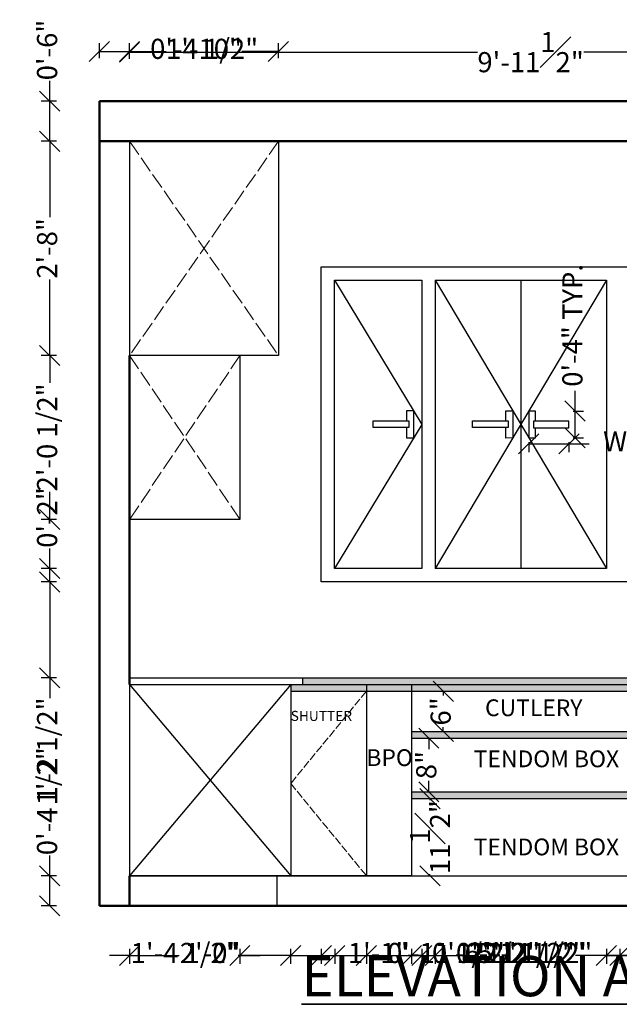
# Model space of a CAD drawing. Units: inches. Extents: x 2164 to 2316, y 625 to 771.
# Tile 1 of 2: x 2164 to 2253, y 625 to 771. Entities that reach past the tile are written whole.
import ezdxf

# ---------------------------------------------------------------- set-up
doc = ezdxf.new("R2010")
doc.units = ezdxf.units.IN
doc.linetypes.add('ACAD_ISO02W100', pattern=[15, 12, -3])
for name, color, linetype, lineweight in [('A-ANNO-DIMS', 2, 'Continuous', 18), ('A-ANNO-TEXT', 7, 'Continuous', 18), ('A-ANNO-TTLB', 7, 'Continuous', 35), ('A-FURN', 30, 'Continuous', 25), ('A-FURN-OPEN', 8, 'ACAD_ISO02W100', 13), ('A-FURN-PATT', 8, 'Continuous', 13), ('A-GLAZ', 4, 'Continuous', 25), ('A-WALL', 7, 'Continuous', 50)]:
    doc.layers.add(name, color=color, linetype=linetype, lineweight=lineweight)
doc.styles.get("Standard").update_dxf_attribs({"font": 'arial.ttf'})
doc.dimstyles.new('ISO-25', dxfattribs={"dimtxt": 3, "dimasz": 3, "dimexe": 1.25, "dimexo": 0.625, "dimtad": 0, "dimdec": 5, "dimlunit": 4, "dimtxsty": 'Standard', "dimblk": 'OBLIQUE', "dimcen": 2.5, "dimclrt": 1, "dimadec": 0, "dimazin": 0, "dimtfac": 1, "dimtdec": 5, "dimtmove": 0, "dimatfit": 3, "dimldrblk": 'OBLIQUE', "dimfxl": 1, "dimfxlon": 1, "dimfrac": 1, "dimarcsym": 0})

# ---------------------------------------------------------------- blocks, each defined once
blk = doc.blocks.new('_Oblique')
at = {"color": 0, "linetype": 'ByBlock', "lineweight": -2}
blk.add_line((-0.5, -0.5), (0.5, 0.5), dxfattribs=at)
blk = doc.blocks.new('*D1')
at = {"layer": 'A-ANNO-DIMS', "color": 0, "lineweight": -2, "transparency": 16777216}
for p, q in [((2226.19, 671.25), (2228.44, 671.25)), ((2227.19, 671.25), (2227.19, 670.61)), ((2226.19, 665.25), (2228.44, 665.25)), ((2227.19, 665.25), (2227.19, 665.9))]:
    blk.add_line(p, q, dxfattribs=at)
at = {"layer": 'Defpoints', "color": 0, "transparency": 16777216}
for p in [(2222.45, 671.25), (2222.45, 665.25), (2227.19, 665.25)]:
    blk.add_point(p, dxfattribs=at)
at = {"layer": 'A-ANNO-DIMS', "color": 0, "lineweight": -2, "transparency": 16777216, "xscale": 3, "yscale": 3, "zscale": 3}
for p, rotation in [((2227.19, 671.25), 90), ((2227.19, 665.25), 270)]:
    blk.add_blockref('_Oblique', p, dxfattribs=dict(at, rotation=rotation))
at = {"layer": 'A-ANNO-DIMS', "color": 0, "transparency": 16777216, "insert": (2227.19, 668.25), "char_height": 3, "attachment_point": 5, "rotation": 90}
blk.add_mtext('6"', dxfattribs=at)
blk = doc.blocks.new('*D2')
at = {"layer": 'A-ANNO-DIMS', "color": 0, "lineweight": -2, "transparency": 16777216}
for p, q in [((2224.04, 664.25), (2226.29, 664.25)), ((2225.04, 664.25), (2225.04, 662.6)), ((2225.04, 656.25), (2225.04, 657.9)), ((2224.04, 656.25), (2226.29, 656.25))]:
    blk.add_line(p, q, dxfattribs=at)
at = {"layer": 'Defpoints', "color": 0, "transparency": 16777216}
for p in [(2222.45, 664.25), (2222.45, 656.25), (2225.04, 656.25)]:
    blk.add_point(p, dxfattribs=at)
at = {"layer": 'A-ANNO-DIMS', "color": 0, "lineweight": -2, "transparency": 16777216, "xscale": 3, "yscale": 3, "zscale": 3}
for p, rotation in [((2225.04, 664.25), 90), ((2225.04, 656.25), 270)]:
    blk.add_blockref('_Oblique', p, dxfattribs=dict(at, rotation=rotation))
at = {"layer": 'A-ANNO-DIMS', "color": 0, "transparency": 16777216, "insert": (2225.04, 660.25), "char_height": 3, "attachment_point": 5, "rotation": 90}
blk.add_mtext('8"', dxfattribs=at)
blk = doc.blocks.new('*D3')
at = {"layer": 'A-ANNO-DIMS', "color": 0, "lineweight": -2, "transparency": 16777216}
for p, q in [((2224.21, 655.25), (2226.46, 655.25)), ((2225.21, 655.25), (2225.21, 655.02)), ((2224.21, 643.75), (2226.46, 643.75)), ((2225.21, 643.75), (2225.21, 643.98))]:
    blk.add_line(p, q, dxfattribs=at)
at = {"layer": 'Defpoints', "color": 0, "transparency": 16777216}
for p in [(2222.45, 655.25), (2222.45, 643.75), (2225.21, 643.75)]:
    blk.add_point(p, dxfattribs=at)
at = {"layer": 'A-ANNO-DIMS', "color": 0, "lineweight": -2, "transparency": 16777216, "xscale": 3, "yscale": 3, "zscale": 3}
for p, rotation in [((2225.21, 655.25), 90), ((2225.21, 643.75), 270)]:
    blk.add_blockref('_Oblique', p, dxfattribs=dict(at, rotation=rotation))
at = {"layer": 'A-ANNO-DIMS', "color": 0, "transparency": 16777216, "insert": (2225.21, 649.5), "char_height": 3, "attachment_point": 5, "rotation": 90}
blk.add_mtext('11{\\H1x;\\S1#2;}"', dxfattribs=at)
blk = doc.blocks.new('*D4')
at = {"layer": 'A-ANNO-DIMS', "color": 0, "lineweight": -2, "transparency": 16777216}
for p, q in [((2180.45, 765.55), (2180.45, 767.8)), ((2299.95, 765.55), (2299.95, 767.8)), ((2180.45, 766.55), (2232.28, 766.55)), ((2299.95, 766.55), (2248.13, 766.55))]:
    blk.add_line(p, q, dxfattribs=at)
at = {"layer": 'Defpoints', "color": 0, "transparency": 16777216}
for p in [(2299.95, 766.55), (2180.45, 759.25), (2299.95, 759.25)]:
    blk.add_point(p, dxfattribs=at)
at = {"layer": 'A-ANNO-DIMS', "color": 0, "lineweight": -2, "transparency": 16777216, "xscale": 3, "yscale": 3, "zscale": 3, "rotation": 180}
blk.add_blockref('_Oblique', (2180.45, 766.55), dxfattribs=at)
at = {"layer": 'A-ANNO-DIMS', "color": 0, "lineweight": -2, "transparency": 16777216, "xscale": 3, "yscale": 3, "zscale": 3}
blk.add_blockref('_Oblique', (2299.95, 766.55), dxfattribs=at)
at = {"layer": 'A-ANNO-DIMS', "color": 0, "transparency": 16777216, "insert": (2240.2, 766.55), "char_height": 3, "attachment_point": 5}
blk.add_mtext('9\'-11{\\H1x;\\S1#2;}"', dxfattribs=at)
blk = doc.blocks.new('WIN-HANDLE')
blk.add_lwpolyline([(2239.92, 710.04), (2239.92, 709.04), (2240.92, 709.04), (2240.92, 710.54), (2245.92, 710.54), (2245.92, 711.54), (2240.92, 711.54), (2240.92, 713.04), (2239.92, 713.04), (2239.92, 711.04)], close=True)
blk.add_lwpolyline([(2240.92, 711.54), (2240.62, 711.54), (2240.62, 710.54), (2240.92, 710.54)])
blk = doc.blocks.new('*D8')
at = {"layer": 'A-ANNO-DIMS', "color": 0, "lineweight": -2, "transparency": 16777216}
for p, q in [((2239.92, 708.42), (2239.92, 706.89)), ((2239.92, 708.14), (2245.92, 708.14)), ((2245.92, 708.42), (2245.92, 706.89)), ((2245.92, 708.14), (2248.92, 708.14))]:
    blk.add_line(p, q, dxfattribs=at)
at = {"layer": 'Defpoints', "color": 0, "transparency": 16777216}
for p in [(2239.92, 709.04), (2245.92, 709.04), (2245.92, 708.14)]:
    blk.add_point(p, dxfattribs=at)
at = {"layer": 'A-ANNO-DIMS', "color": 0, "lineweight": -2, "transparency": 16777216, "xscale": 3, "yscale": 3, "zscale": 3, "rotation": 180}
blk.add_blockref('_Oblique', (2239.92, 708.14), dxfattribs=at)
at = {"layer": 'A-ANNO-DIMS', "color": 0, "lineweight": -2, "transparency": 16777216, "xscale": 3, "yscale": 3, "zscale": 3}
blk.add_blockref('_Oblique', (2245.92, 708.14), dxfattribs=at)
at = {"layer": 'A-ANNO-DIMS', "color": 1, "transparency": 16777216, "insert": (2277.61, 708.14), "char_height": 3, "attachment_point": 5}
blk.add_mtext('WINDOW HANDLE 0\'-6" TYP.', dxfattribs=at)
blk = doc.blocks.new('*D9')
at = {"layer": 'A-ANNO-DIMS', "color": 0, "lineweight": -2, "transparency": 16777216}
for p, q in [((2246.82, 713.04), (2246.82, 716.04)), ((2246.55, 713.04), (2248.07, 713.04)), ((2246.82, 709.04), (2246.82, 713.04)), ((2246.55, 709.04), (2248.07, 709.04))]:
    blk.add_line(p, q, dxfattribs=at)
at = {"layer": 'Defpoints', "color": 0, "transparency": 16777216}
for p in [(2245.92, 713.04), (2246.82, 713.04), (2245.92, 709.04)]:
    blk.add_point(p, dxfattribs=at)
at = {"layer": 'A-ANNO-DIMS', "color": 0, "lineweight": -2, "transparency": 16777216, "xscale": 3, "yscale": 3, "zscale": 3}
for p, rotation in [((2246.82, 713.04), 90), ((2246.82, 709.04), 270)]:
    blk.add_blockref('_Oblique', p, dxfattribs=dict(at, rotation=rotation))
at = {"layer": 'A-ANNO-DIMS', "color": 1, "transparency": 16777216, "insert": (2246.82, 725.81), "char_height": 3, "attachment_point": 5, "rotation": 90}
blk.add_mtext('0\'-4" TYP.', dxfattribs=at)
blk = doc.blocks.new('*D10')
at = {"layer": 'A-ANNO-DIMS', "color": 0, "lineweight": -2, "transparency": 16777216}
for p, q in [((2180.45, 765.65), (2180.45, 767.9)), ((2202.62, 765.65), (2202.62, 767.9)), ((2180.45, 766.65), (2185.9, 766.65)), ((2202.62, 766.65), (2197.17, 766.65))]:
    blk.add_line(p, q, dxfattribs=at)
at = {"layer": 'Defpoints', "color": 0, "transparency": 16777216}
for p in [(2202.62, 766.65), (2180.45, 753.25), (2202.62, 753.25)]:
    blk.add_point(p, dxfattribs=at)
at = {"layer": 'A-ANNO-DIMS', "color": 0, "lineweight": -2, "transparency": 16777216, "xscale": 3, "yscale": 3, "zscale": 3, "rotation": 180}
blk.add_blockref('_Oblique', (2180.45, 766.65), dxfattribs=at)
at = {"layer": 'A-ANNO-DIMS', "color": 0, "lineweight": -2, "transparency": 16777216, "xscale": 3, "yscale": 3, "zscale": 3}
blk.add_blockref('_Oblique', (2202.62, 766.65), dxfattribs=at)
at = {"layer": 'A-ANNO-DIMS', "color": 1, "transparency": 16777216, "insert": (2191.54, 766.65), "char_height": 3, "attachment_point": 5}
blk.add_mtext('1\'-10"', dxfattribs=at)
blk = doc.blocks.new('*D12')
at = {"layer": 'A-ANNO-DIMS', "color": 0, "lineweight": -2, "transparency": 16777216}
for p, q in [((2169.55, 753.25), (2167.3, 753.25)), ((2168.55, 753.25), (2168.55, 741.93)), ((2168.55, 721.33), (2168.55, 732.65)), ((2169.55, 721.33), (2167.3, 721.33))]:
    blk.add_line(p, q, dxfattribs=at)
at = {"layer": 'Defpoints', "color": 0, "transparency": 16777216}
for p in [(2180.45, 753.25), (2168.55, 721.33), (2180.45, 721.33)]:
    blk.add_point(p, dxfattribs=at)
at = {"layer": 'A-ANNO-DIMS', "color": 0, "lineweight": -2, "transparency": 16777216, "xscale": 3, "yscale": 3, "zscale": 3}
for p, rotation in [((2168.55, 753.25), 90), ((2168.55, 721.33), 270)]:
    blk.add_blockref('_Oblique', p, dxfattribs=dict(at, rotation=rotation))
at = {"layer": 'A-ANNO-DIMS', "color": 1, "transparency": 16777216, "insert": (2168.55, 737.29), "char_height": 3, "attachment_point": 5, "rotation": 90}
blk.add_mtext('2\'-8"', dxfattribs=at)
blk = doc.blocks.new('*D13')
at = {"layer": 'A-ANNO-DIMS', "color": 0, "lineweight": -2, "transparency": 16777216}
for p, q in [((2169.55, 721.33), (2167.3, 721.33)), ((2168.55, 721.33), (2168.55, 717.24)), ((2168.55, 696.88), (2168.55, 700.97)), ((2169.55, 696.88), (2167.3, 696.88))]:
    blk.add_line(p, q, dxfattribs=at)
at = {"layer": 'Defpoints', "color": 0, "transparency": 16777216}
for p in [(2180.45, 721.33), (2168.55, 696.88), (2180.45, 696.88)]:
    blk.add_point(p, dxfattribs=at)
at = {"layer": 'A-ANNO-DIMS', "color": 0, "lineweight": -2, "transparency": 16777216, "xscale": 3, "yscale": 3, "zscale": 3}
for p, rotation in [((2168.55, 721.33), 90), ((2168.55, 696.88), 270)]:
    blk.add_blockref('_Oblique', p, dxfattribs=dict(at, rotation=rotation))
at = {"layer": 'A-ANNO-DIMS', "color": 1, "transparency": 16777216, "insert": (2168.55, 709.11), "char_height": 3, "attachment_point": 5, "rotation": 90}
blk.add_mtext('2\'-0 1/2"', dxfattribs=at)
blk = doc.blocks.new('*D14')
at = {"layer": 'A-ANNO-DIMS', "color": 0, "lineweight": -2, "transparency": 16777216}
for p, q in [((2180.45, 632.85), (2180.45, 630.6)), ((2196.89, 632.85), (2196.89, 630.6)), ((2180.45, 631.85), (2177.45, 631.85)), ((2180.45, 631.85), (2180.71, 631.85)), ((2196.89, 631.85), (2196.64, 631.85)), ((2196.89, 631.85), (2199.89, 631.85))]:
    blk.add_line(p, q, dxfattribs=at)
at = {"layer": 'Defpoints', "color": 0, "transparency": 16777216}
for p in [(2180.45, 696.88), (2196.89, 696.88), (2196.89, 631.85)]:
    blk.add_point(p, dxfattribs=at)
at = {"layer": 'A-ANNO-DIMS', "color": 0, "lineweight": -2, "transparency": 16777216, "xscale": 3, "yscale": 3, "zscale": 3}
blk.add_blockref('_Oblique', (2180.45, 631.85), dxfattribs=at)
at = {"layer": 'A-ANNO-DIMS', "color": 0, "lineweight": -2, "transparency": 16777216, "xscale": 3, "yscale": 3, "zscale": 3, "rotation": 180}
blk.add_blockref('_Oblique', (2196.89, 631.85), dxfattribs=at)
at = {"layer": 'A-ANNO-DIMS', "color": 1, "transparency": 16777216, "insert": (2188.67, 631.85), "char_height": 3, "attachment_point": 5}
blk.add_mtext('1\'-4 1/2"', dxfattribs=at)
blk = doc.blocks.new('*D17')
at = {"layer": 'A-ANNO-DIMS', "color": 0, "lineweight": -2, "transparency": 16777216}
for p, q in [((2211.01, 632.85), (2211.01, 630.6)), ((2223.98, 632.85), (2223.98, 630.6)), ((2211.01, 631.85), (2213.02, 631.85)), ((2223.98, 631.85), (2221.96, 631.85))]:
    blk.add_line(p, q, dxfattribs=at)
at = {"layer": 'Defpoints', "color": 0, "transparency": 16777216}
for p in [(2211.01, 689.55), (2223.98, 689.55), (2223.98, 631.85)]:
    blk.add_point(p, dxfattribs=at)
at = {"layer": 'A-ANNO-DIMS', "color": 0, "lineweight": -2, "transparency": 16777216, "xscale": 3, "yscale": 3, "zscale": 3, "rotation": 180}
blk.add_blockref('_Oblique', (2211.01, 631.85), dxfattribs=at)
at = {"layer": 'A-ANNO-DIMS', "color": 0, "lineweight": -2, "transparency": 16777216, "xscale": 3, "yscale": 3, "zscale": 3}
blk.add_blockref('_Oblique', (2223.98, 631.85), dxfattribs=at)
at = {"layer": 'A-ANNO-DIMS', "color": 1, "transparency": 16777216, "insert": (2217.49, 631.85), "char_height": 3, "attachment_point": 5}
blk.add_mtext('1\'-1"', dxfattribs=at)
blk = doc.blocks.new('*D18')
at = {"layer": 'A-ANNO-DIMS', "color": 0, "lineweight": -2, "transparency": 16777216}
for p, q in [((2223.98, 632.85), (2223.98, 630.6)), ((2225.98, 632.85), (2225.98, 630.6)), ((2223.98, 631.85), (2225.98, 631.85)), ((2225.98, 631.85), (2228.98, 631.85))]:
    blk.add_line(p, q, dxfattribs=at)
at = {"layer": 'Defpoints', "color": 0, "transparency": 16777216}
for p in [(2223.98, 689.55), (2225.98, 689.55), (2225.98, 631.85)]:
    blk.add_point(p, dxfattribs=at)
at = {"layer": 'A-ANNO-DIMS', "color": 0, "lineweight": -2, "transparency": 16777216, "xscale": 3, "yscale": 3, "zscale": 3, "rotation": 180}
blk.add_blockref('_Oblique', (2223.98, 631.85), dxfattribs=at)
at = {"layer": 'A-ANNO-DIMS', "color": 0, "lineweight": -2, "transparency": 16777216, "xscale": 3, "yscale": 3, "zscale": 3}
blk.add_blockref('_Oblique', (2225.98, 631.85), dxfattribs=at)
at = {"layer": 'A-ANNO-DIMS', "color": 1, "transparency": 16777216, "insert": (2233.59, 631.85), "char_height": 3, "attachment_point": 5}
blk.add_mtext('0\'-2"', dxfattribs=at)
blk = doc.blocks.new('*D19')
at = {"layer": 'A-ANNO-DIMS', "color": 0, "lineweight": -2, "transparency": 16777216}
for p, q in [((2225.98, 632.85), (2225.98, 630.6)), ((2251.49, 632.85), (2251.49, 630.6)), ((2225.98, 631.85), (2230.6, 631.85)), ((2251.49, 631.85), (2246.87, 631.85))]:
    blk.add_line(p, q, dxfattribs=at)
at = {"layer": 'Defpoints', "color": 0, "transparency": 16777216}
for p in [(2225.98, 689.55), (2251.49, 689.55), (2251.49, 631.85)]:
    blk.add_point(p, dxfattribs=at)
at = {"layer": 'A-ANNO-DIMS', "color": 0, "lineweight": -2, "transparency": 16777216, "xscale": 3, "yscale": 3, "zscale": 3, "rotation": 180}
blk.add_blockref('_Oblique', (2225.98, 631.85), dxfattribs=at)
at = {"layer": 'A-ANNO-DIMS', "color": 0, "lineweight": -2, "transparency": 16777216, "xscale": 3, "yscale": 3, "zscale": 3}
blk.add_blockref('_Oblique', (2251.49, 631.85), dxfattribs=at)
at = {"layer": 'A-ANNO-DIMS', "color": 1, "transparency": 16777216, "insert": (2238.74, 631.85), "char_height": 3, "attachment_point": 5}
blk.add_mtext('2\'-1 1/2"', dxfattribs=at)
blk = doc.blocks.new('*D20')
at = {"layer": 'A-ANNO-DIMS', "color": 0, "lineweight": -2, "transparency": 16777216}
for p, q in [((2251.49, 632.85), (2251.49, 630.6)), ((2253.49, 632.85), (2253.49, 630.6)), ((2251.49, 631.85), (2253.49, 631.85)), ((2253.49, 631.85), (2256.49, 631.85))]:
    blk.add_line(p, q, dxfattribs=at)
at = {"layer": 'Defpoints', "color": 0, "transparency": 16777216}
for p in [(2251.49, 689.55), (2253.49, 689.55), (2253.49, 631.85)]:
    blk.add_point(p, dxfattribs=at)
at = {"layer": 'A-ANNO-DIMS', "color": 0, "lineweight": -2, "transparency": 16777216, "xscale": 3, "yscale": 3, "zscale": 3, "rotation": 180}
blk.add_blockref('_Oblique', (2251.49, 631.85), dxfattribs=at)
at = {"layer": 'A-ANNO-DIMS', "color": 0, "lineweight": -2, "transparency": 16777216, "xscale": 3, "yscale": 3, "zscale": 3}
blk.add_blockref('_Oblique', (2253.49, 631.85), dxfattribs=at)
at = {"layer": 'A-ANNO-DIMS', "color": 1, "transparency": 16777216, "insert": (2261.11, 631.85), "char_height": 3, "attachment_point": 5}
blk.add_mtext('0\'-2"', dxfattribs=at)
blk = doc.blocks.new('*D21')
at = {"layer": 'A-ANNO-DIMS', "color": 0, "lineweight": -2, "transparency": 16777216}
for p, q in [((2253.49, 632.85), (2253.49, 630.6)), ((2269.66, 632.85), (2269.66, 630.6)), ((2253.49, 631.85), (2257.11, 631.85)), ((2269.66, 631.85), (2266.05, 631.85))]:
    blk.add_line(p, q, dxfattribs=at)
at = {"layer": 'Defpoints', "color": 0, "transparency": 16777216}
for p in [(2253.49, 689.55), (2269.66, 689.55), (2269.66, 631.85)]:
    blk.add_point(p, dxfattribs=at)
at = {"layer": 'A-ANNO-DIMS', "color": 0, "lineweight": -2, "transparency": 16777216, "xscale": 3, "yscale": 3, "zscale": 3, "rotation": 180}
blk.add_blockref('_Oblique', (2253.49, 631.85), dxfattribs=at)
at = {"layer": 'A-ANNO-DIMS', "color": 0, "lineweight": -2, "transparency": 16777216, "xscale": 3, "yscale": 3, "zscale": 3}
blk.add_blockref('_Oblique', (2269.66, 631.85), dxfattribs=at)
at = {"layer": 'A-ANNO-DIMS', "color": 1, "transparency": 16777216, "insert": (2261.58, 631.85), "char_height": 3, "attachment_point": 5}
blk.add_mtext('1\'-4"', dxfattribs=at)
blk = doc.blocks.new('*D23')
at = {"layer": 'A-ANNO-DIMS', "color": 0, "lineweight": -2, "transparency": 16777216}
for p, q in [((2209.01, 632.85), (2209.01, 630.6)), ((2271.66, 632.85), (2271.66, 630.6)), ((2209.01, 631.85), (2232.23, 631.85)), ((2271.66, 631.85), (2248.44, 631.85))]:
    blk.add_line(p, q, dxfattribs=at)
at = {"layer": 'Defpoints', "color": 0, "transparency": 16777216}
for p in [(2209.01, 687.55), (2271.66, 687.55), (2271.66, 631.85)]:
    blk.add_point(p, dxfattribs=at)
at = {"layer": 'A-ANNO-DIMS', "color": 0, "lineweight": -2, "transparency": 16777216, "xscale": 3, "yscale": 3, "zscale": 3, "rotation": 180}
blk.add_blockref('_Oblique', (2209.01, 631.85), dxfattribs=at)
at = {"layer": 'A-ANNO-DIMS', "color": 0, "lineweight": -2, "transparency": 16777216, "xscale": 3, "yscale": 3, "zscale": 3}
blk.add_blockref('_Oblique', (2271.66, 631.85), dxfattribs=at)
at = {"layer": 'A-ANNO-DIMS', "color": 1, "transparency": 16777216, "insert": (2240.33, 631.85), "char_height": 3, "attachment_point": 5}
blk.add_mtext('5\'-2 1/2"', dxfattribs=at)
blk = doc.blocks.new('*D25')
at = {"layer": 'A-ANNO-DIMS', "color": 0, "lineweight": -2, "transparency": 16777216}
for p, q in [((2168.55, 689.55), (2168.55, 692.55)), ((2169.55, 689.55), (2167.3, 689.55)), ((2168.55, 687.55), (2168.55, 689.55)), ((2169.55, 687.55), (2167.3, 687.55))]:
    blk.add_line(p, q, dxfattribs=at)
at = {"layer": 'Defpoints', "color": 0, "transparency": 16777216}
for p in [(2168.55, 689.55), (2211.01, 689.55), (2209.01, 687.55)]:
    blk.add_point(p, dxfattribs=at)
at = {"layer": 'A-ANNO-DIMS', "color": 0, "lineweight": -2, "transparency": 16777216, "xscale": 3, "yscale": 3, "zscale": 3}
for p, rotation in [((2168.55, 689.55), 90), ((2168.55, 687.55), 270)]:
    blk.add_blockref('_Oblique', p, dxfattribs=dict(at, rotation=rotation))
at = {"layer": 'A-ANNO-DIMS', "color": 1, "transparency": 16777216, "insert": (2168.55, 697.16), "char_height": 3, "attachment_point": 5, "rotation": 90}
blk.add_mtext('0\'-2"', dxfattribs=at)
blk = doc.blocks.new('*D29')
at = {"layer": 'A-ANNO-DIMS', "color": 0, "lineweight": -2, "transparency": 16777216}
for p, q in [((2169.55, 687.55), (2167.3, 687.55)), ((2168.55, 687.55), (2168.55, 673.25)), ((2169.55, 673.25), (2167.3, 673.25)), ((2168.55, 673.25), (2168.55, 670.25))]:
    blk.add_line(p, q, dxfattribs=at)
at = {"layer": 'Defpoints', "color": 0, "transparency": 16777216}
for p in [(2209.01, 687.55), (2168.55, 673.25), (2180.45, 673.25)]:
    blk.add_point(p, dxfattribs=at)
at = {"layer": 'A-ANNO-DIMS', "color": 0, "lineweight": -2, "transparency": 16777216, "xscale": 3, "yscale": 3, "zscale": 3}
for p, rotation in [((2168.55, 687.55), 90), ((2168.55, 673.25), 270)]:
    blk.add_blockref('_Oblique', p, dxfattribs=dict(at, rotation=rotation))
at = {"layer": 'A-ANNO-DIMS', "color": 1, "transparency": 16777216, "insert": (2168.55, 662.29), "char_height": 3, "attachment_point": 5, "rotation": 90}
blk.add_mtext('1\'-2 1/2"', dxfattribs=at)
blk = doc.blocks.new('*D34')
at = {"layer": 'A-ANNO-DIMS', "color": 0, "lineweight": -2, "transparency": 16777216}
for p, q in [((2168.55, 643.75), (2168.55, 646.75)), ((2169.55, 643.75), (2167.3, 643.75)), ((2168.55, 639.25), (2168.55, 643.75)), ((2169.55, 639.25), (2167.3, 639.25))]:
    blk.add_line(p, q, dxfattribs=at)
at = {"layer": 'Defpoints', "color": 0, "transparency": 16777216}
for p in [(2168.55, 643.75), (2180.45, 643.75), (2180.45, 639.25)]:
    blk.add_point(p, dxfattribs=at)
at = {"layer": 'A-ANNO-DIMS', "color": 0, "lineweight": -2, "transparency": 16777216, "xscale": 3, "yscale": 3, "zscale": 3}
for p, rotation in [((2168.55, 643.75), 90), ((2168.55, 639.25), 270)]:
    blk.add_blockref('_Oblique', p, dxfattribs=dict(at, rotation=rotation))
at = {"layer": 'A-ANNO-DIMS', "color": 1, "transparency": 16777216, "insert": (2168.55, 654.86), "char_height": 3, "attachment_point": 5, "rotation": 90}
blk.add_mtext('0\'-4 1/2"', dxfattribs=at)
blk = doc.blocks.new('*D35')
at = {"layer": 'A-ANNO-DIMS', "color": 0, "lineweight": -2, "transparency": 16777216}
for p, q in [((2180.45, 632.85), (2180.45, 630.6)), ((2204.45, 632.85), (2204.45, 630.6)), ((2180.45, 631.85), (2187.82, 631.85)), ((2204.45, 631.85), (2197.09, 631.85))]:
    blk.add_line(p, q, dxfattribs=at)
at = {"layer": 'Defpoints', "color": 0, "transparency": 16777216}
for p in [(2180.45, 643.75), (2204.45, 643.75), (2204.45, 631.85)]:
    blk.add_point(p, dxfattribs=at)
at = {"layer": 'A-ANNO-DIMS', "color": 0, "lineweight": -2, "transparency": 16777216, "xscale": 3, "yscale": 3, "zscale": 3, "rotation": 180}
blk.add_blockref('_Oblique', (2180.45, 631.85), dxfattribs=at)
at = {"layer": 'A-ANNO-DIMS', "color": 0, "lineweight": -2, "transparency": 16777216, "xscale": 3, "yscale": 3, "zscale": 3}
blk.add_blockref('_Oblique', (2204.45, 631.85), dxfattribs=at)
at = {"layer": 'A-ANNO-DIMS', "color": 1, "transparency": 16777216, "insert": (2192.45, 631.85), "char_height": 3, "attachment_point": 5}
blk.add_mtext('2\'-0"', dxfattribs=at)
blk = doc.blocks.new('*D36')
at = {"layer": 'A-ANNO-DIMS', "color": 0, "lineweight": -2, "transparency": 16777216}
for p, q in [((2204.45, 632.85), (2204.45, 630.6)), ((2215.73, 632.85), (2215.73, 630.6)), ((2204.45, 631.85), (2215.73, 631.85)), ((2215.73, 631.85), (2218.73, 631.85))]:
    blk.add_line(p, q, dxfattribs=at)
at = {"layer": 'Defpoints', "color": 0, "transparency": 16777216}
for p in [(2204.45, 643.75), (2215.73, 643.75), (2215.73, 631.85)]:
    blk.add_point(p, dxfattribs=at)
at = {"layer": 'A-ANNO-DIMS', "color": 0, "lineweight": -2, "transparency": 16777216, "xscale": 3, "yscale": 3, "zscale": 3, "rotation": 180}
blk.add_blockref('_Oblique', (2204.45, 631.85), dxfattribs=at)
at = {"layer": 'A-ANNO-DIMS', "color": 0, "lineweight": -2, "transparency": 16777216, "xscale": 3, "yscale": 3, "zscale": 3}
blk.add_blockref('_Oblique', (2215.73, 631.85), dxfattribs=at)
at = {"layer": 'A-ANNO-DIMS', "color": 1, "transparency": 16777216, "insert": (2228, 631.85), "char_height": 3, "attachment_point": 5}
blk.add_mtext('0\'-11 1/2"', dxfattribs=at)
blk = doc.blocks.new('*D37')
at = {"layer": 'A-ANNO-DIMS', "color": 0, "lineweight": -2, "transparency": 16777216}
for p, q in [((2215.73, 632.85), (2215.73, 630.6)), ((2222.45, 632.85), (2222.45, 630.6)), ((2215.73, 631.85), (2222.45, 631.85)), ((2222.45, 631.85), (2225.45, 631.85))]:
    blk.add_line(p, q, dxfattribs=at)
at = {"layer": 'Defpoints', "color": 0, "transparency": 16777216}
for p in [(2215.73, 643.75), (2222.45, 643.75), (2222.45, 631.85)]:
    blk.add_point(p, dxfattribs=at)
at = {"layer": 'A-ANNO-DIMS', "color": 0, "lineweight": -2, "transparency": 16777216, "xscale": 3, "yscale": 3, "zscale": 3, "rotation": 180}
blk.add_blockref('_Oblique', (2215.73, 631.85), dxfattribs=at)
at = {"layer": 'A-ANNO-DIMS', "color": 0, "lineweight": -2, "transparency": 16777216, "xscale": 3, "yscale": 3, "zscale": 3}
blk.add_blockref('_Oblique', (2222.45, 631.85), dxfattribs=at)
at = {"layer": 'A-ANNO-DIMS', "color": 1, "transparency": 16777216, "insert": (2233.56, 631.85), "char_height": 3, "attachment_point": 5}
blk.add_mtext('0\'-6 1/2"', dxfattribs=at)
blk = doc.blocks.new('*D38')
at = {"layer": 'A-ANNO-DIMS', "color": 0, "lineweight": -2, "transparency": 16777216}
for p, q in [((2222.45, 632.85), (2222.45, 630.6)), ((2257.95, 632.85), (2257.95, 630.6)), ((2222.45, 631.85), (2230.9, 631.85)), ((2257.95, 631.85), (2249.5, 631.85))]:
    blk.add_line(p, q, dxfattribs=at)
at = {"layer": 'Defpoints', "color": 0, "transparency": 16777216}
for p in [(2222.45, 643.75), (2257.95, 643.75), (2257.95, 631.85)]:
    blk.add_point(p, dxfattribs=at)
at = {"layer": 'A-ANNO-DIMS', "color": 0, "lineweight": -2, "transparency": 16777216, "xscale": 3, "yscale": 3, "zscale": 3, "rotation": 180}
blk.add_blockref('_Oblique', (2222.45, 631.85), dxfattribs=at)
at = {"layer": 'A-ANNO-DIMS', "color": 0, "lineweight": -2, "transparency": 16777216, "xscale": 3, "yscale": 3, "zscale": 3}
blk.add_blockref('_Oblique', (2257.95, 631.85), dxfattribs=at)
at = {"layer": 'A-ANNO-DIMS', "color": 1, "transparency": 16777216, "insert": (2240.2, 631.85), "char_height": 3, "attachment_point": 5}
blk.add_mtext('2\'-11 1/2"', dxfattribs=at)
blk = doc.blocks.new('*D41')
at = {"layer": 'A-ANNO-DIMS', "color": 0, "lineweight": -2, "transparency": 16777216}
for p, q in [((2175.95, 765.65), (2175.95, 767.9)), ((2180.45, 765.65), (2180.45, 767.9)), ((2175.95, 766.65), (2180.45, 766.65)), ((2180.45, 766.65), (2183.45, 766.65))]:
    blk.add_line(p, q, dxfattribs=at)
at = {"layer": 'Defpoints', "color": 0, "transparency": 16777216}
for p in [(2180.45, 766.65), (2175.95, 759.25), (2180.45, 753.25)]:
    blk.add_point(p, dxfattribs=at)
at = {"layer": 'A-ANNO-DIMS', "color": 0, "lineweight": -2, "transparency": 16777216, "xscale": 3, "yscale": 3, "zscale": 3, "rotation": 180}
blk.add_blockref('_Oblique', (2175.95, 766.65), dxfattribs=at)
at = {"layer": 'A-ANNO-DIMS', "color": 0, "lineweight": -2, "transparency": 16777216, "xscale": 3, "yscale": 3, "zscale": 3}
blk.add_blockref('_Oblique', (2180.45, 766.65), dxfattribs=at)
at = {"layer": 'A-ANNO-DIMS', "color": 1, "transparency": 16777216, "insert": (2191.56, 766.65), "char_height": 3, "attachment_point": 5}
blk.add_mtext('0\'-4 1/2"', dxfattribs=at)
blk = doc.blocks.new('*D42')
at = {"layer": 'A-ANNO-DIMS', "color": 0, "lineweight": -2, "transparency": 16777216}
for p, q in [((2168.55, 759.25), (2168.55, 762.25)), ((2169.55, 759.25), (2167.3, 759.25)), ((2168.55, 753.25), (2168.55, 759.25)), ((2169.55, 753.25), (2167.3, 753.25))]:
    blk.add_line(p, q, dxfattribs=at)
at = {"layer": 'Defpoints', "color": 0, "transparency": 16777216}
for p in [(2168.55, 759.25), (2175.95, 759.25), (2175.95, 753.25)]:
    blk.add_point(p, dxfattribs=at)
at = {"layer": 'A-ANNO-DIMS', "color": 0, "lineweight": -2, "transparency": 16777216, "xscale": 3, "yscale": 3, "zscale": 3}
for p, rotation in [((2168.55, 759.25), 90), ((2168.55, 753.25), 270)]:
    blk.add_blockref('_Oblique', p, dxfattribs=dict(at, rotation=rotation))
at = {"layer": 'A-ANNO-DIMS', "color": 1, "transparency": 16777216, "insert": (2168.55, 766.87), "char_height": 3, "attachment_point": 5, "rotation": 90}
blk.add_mtext('0\'-6"', dxfattribs=at)

msp = doc.modelspace()

# ---------------------------------------------------------------- hatches: boundary and pattern name
at = {"layer": 'A-FURN-PATT'}
h = msp.add_hatch(color=256, dxfattribs=at)
h.dxf.hatch_style = 1
h.paths.add_polyline_path([(2274.687404, 673.253049), (2206.256774, 673.253049), (2206.256774, 672.253049), (2222.453229, 672.253049), (2257.953229, 672.253049), (2274.687404, 672.253049)])
h = msp.add_hatch(color=256, dxfattribs=at)
h.dxf.hatch_style = 1
h.paths.add_polyline_path([(2257.953229, 672.253049), (2222.453229, 672.253049), (2222.453229, 671.253049), (2257.953229, 671.253049)])
h.paths.add_polyline_path([(2257.953229, 665.253049), (2222.453229, 665.253049), (2222.453229, 664.253049), (2257.953229, 664.253049)])
h.paths.add_polyline_path([(2275.953229, 665.253049), (2257.953229, 665.253049), (2257.953229, 664.253049), (2275.953229, 664.253049)])
h.paths.add_polyline_path([(2257.953229, 656.253049), (2222.453229, 656.253049), (2222.453229, 655.253049), (2257.953229, 655.253049)])
h.paths.add_polyline_path([(2275.953229, 672.253049), (2257.953229, 672.253049), (2257.953229, 671.253049), (2275.953229, 671.253049)])
h.paths.add_polyline_path([(2215.731449, 672.253049), (2204.453229, 672.253049), (2204.453229, 671.253049), (2215.731449, 671.253049)])
h.paths.add_polyline_path([(2222.453229, 672.253049), (2215.731449, 672.253049), (2215.731449, 671.253049), (2222.453229, 671.253049)])

# ---------------------------------------------------------------- linework, layer by layer
at = {"layer": 'A-FURN'}
for p, q in [((2180.453229, 753.253049), (2180.453229, 721.327988)), ((2202.619559, 753.253049), (2202.619559, 721.327988)), ((2202.619559, 721.327988), (2180.453229, 721.327988)), ((2196.891249, 721.327988), (2196.891249, 696.882525)), ((2196.891249, 696.882525), (2180.453229, 696.882525)), ((2180.453229, 673.253049), (2299.953229, 673.253049)), ((2206.256774, 672.253049), (2206.256774, 673.253049)), ((2180.453229, 672.253049), (2204.453229, 672.253049)), ((2180.453229, 672.253049), (2180.453229, 643.753049)), ((2180.453229, 672.253049), (2204.453229, 643.753049)), ((2204.453229, 672.253049), (2180.453229, 643.753049)), ((2204.453229, 672.253049), (2204.453229, 643.753049)), ((2204.453229, 672.253049), (2222.453229, 672.253049)), ((2204.453229, 671.253049), (2275.953229, 671.253049)), ((2215.731449, 672.253049), (2215.731449, 643.753049)), ((2222.453229, 672.253049), (2222.453229, 643.753049)), ((2222.453229, 672.253049), (2257.953229, 672.253049)), ((2222.453229, 665.253049), (2275.953229, 665.253049)), ((2222.453229, 664.253049), (2275.953229, 664.253049)), ((2222.453229, 656.253049), (2257.953229, 656.253049)), ((2222.453229, 655.253049), (2257.953229, 655.253049)), ((2180.453229, 643.753049), (2299.953229, 643.753049)), ((2222.453229, 643.753049), (2180.453229, 643.753049)), ((2202.399179, 643.753049), (2202.399179, 639.253049))]:
    msp.add_line(p, q, dxfattribs=at)
at = {"layer": 'A-FURN-OPEN', "ltscale": 0.2}
for p, q in [((2180.453229, 753.253049), (2202.619559, 721.327988)), ((2202.619559, 753.253049), (2180.453229, 721.327988)), ((2180.453229, 721.327988), (2196.891249, 696.882525)), ((2196.891249, 721.327988), (2180.453229, 696.882525))]:
    msp.add_line(p, q, dxfattribs=at)
at = {"layer": 'A-FURN-OPEN', "ltscale": 0.1}
for p, q in [((2215.731449, 671.253049), (2204.453229, 657.503049)), ((2204.453229, 657.503049), (2215.731449, 643.753049))]:
    msp.add_line(p, q, dxfattribs=at)
at = {"layer": 'A-GLAZ'}
for p, q in [((2211.005798, 732.541226), (2223.976266, 732.541226)), ((2211.005798, 689.550561), (2211.005798, 732.541226)), ((2211.005798, 732.541226), (2223.976266, 711.045894)), ((2223.976266, 732.541226), (2223.976266, 689.550561)), ((2225.976266, 732.541226), (2225.976266, 689.550561)), ((2225.976266, 732.541226), (2251.49409, 732.541226)), ((2225.976266, 732.541226), (2251.49409, 689.550561)), ((2251.49409, 732.541226), (2225.976266, 689.550561)), ((2238.735178, 732.541226), (2238.735178, 689.550561)), ((2251.49409, 732.541226), (2251.49409, 689.550561)), ((2223.976266, 711.045894), (2211.005798, 689.550561)), ((2223.976266, 689.550561), (2211.005798, 689.550561)), ((2251.49409, 689.550561), (2225.976266, 689.550561))]:
    msp.add_line(p, q, dxfattribs=at)
for points in [[(2209.005798, 734.541226), (2271.663741, 734.541226), (2271.663741, 687.550561), (2209.005798, 687.550561)], [(2222.740131, 710.094479), (2222.740131, 709.004004), (2221.740131, 709.004004), (2221.740131, 710.594479), (2216.740131, 710.594479), (2216.740131, 711.594479), (2221.740131, 711.594479), (2221.740131, 713.094479), (2222.740131, 713.094479), (2222.740131, 711.094479)], [(2237.53146, 710.073834), (2237.53146, 709.017953), (2236.53146, 709.011334), (2236.53146, 710.573834), (2231.53146, 710.573834), (2231.53146, 711.573834), (2236.53146, 711.573834), (2236.53146, 713.073834), (2237.53146, 713.073834), (2237.53146, 711.073834)]]:
    msp.add_lwpolyline(points, close=True, dxfattribs=at)
for points in [[(2221.740131, 711.594479), (2222.045344, 711.594479), (2222.045344, 710.594479), (2221.740131, 710.594479)], [(2236.53146, 711.573834), (2236.836673, 711.573834), (2236.836673, 710.573834), (2236.53146, 710.573834)]]:
    msp.add_lwpolyline(points, dxfattribs=at)
at = {"layer": 'A-WALL'}
for p, q in [((2304.453229, 759.253049), (2175.953229, 759.253049)), ((2175.953229, 759.253049), (2175.953229, 639.253049)), ((2304.453229, 753.253049), (2175.953229, 753.253049)), ((2180.453229, 721.327988), (2180.453229, 672.253049)), ((2180.453229, 643.753049), (2180.453229, 639.253049)), ((2175.953229, 639.253049), (2304.453229, 639.253049))]:
    msp.add_line(p, q, dxfattribs=at)

# ---------------------------------------------------------------- block references
at = {"layer": 'A-GLAZ'}
msp.add_blockref('WIN-HANDLE', (0, 0), dxfattribs=at)

# ---------------------------------------------------------------- texts
at = {"layer": 'A-ANNO-TEXT', "attachment_point": 1}
for s, width, insert, char_height in [('CUTLERY', 18.44873395, (2233.410249, 670.043616), 2.5), ('SHUTTER', 10.15014856, (2204.453229, 668.333549), 1.5), ('BPO', 4.08398305, (2215.731449, 662.605635), 2.5), ('TENDOM BOX', 23.78004909, (2231.733024, 662.428607), 2.5), ('TENDOM BOX', 23.78004909, (2231.733024, 649.29578), 2.5)]:
    msp.add_mtext_dynamic_manual_height_columns(s, width=width, gutter_width=12.5, heights=[0], dxfattribs=dict(at, insert=insert, char_height=char_height))
at = {"layer": 'A-ANNO-TTLB', "insert": (2206.044532, 631.780545), "char_height": 6, "attachment_point": 1}
msp.add_mtext_dynamic_manual_height_columns('{\\LELEVATION A}', width=73.64161161, gutter_width=12.5, heights=[0], dxfattribs=at)

# ---------------------------------------------------------------- dimensions: what is measured, and where the dimension line sits
at = {"layer": 'A-ANNO-DIMS'}
for base, p1, p2, override, picture, middle in [((2168.553229, 759.253049), (2175.953229, 753.253049), (2175.953229, 759.253049), {"dimdec": 1, "dimlfac": 1, "dimrnd": 0, "dimzin": 1, "dimdsep": 46, "dimlunit": 4, "dimfrac": 2}, '*D42', (2168.553229, 766.86543)), ((2168.553229, 721.327988), (2180.453229, 753.253049), (2180.453229, 721.327988), {"dimdec": 1, "dimlfac": 1, "dimrnd": 0, "dimzin": 1, "dimdsep": 46, "dimlunit": 4, "dimfrac": 2}, '*D12', (2168.553229, 737.290518)), ((2168.553229, 696.882525), (2180.453229, 721.327988), (2180.453229, 696.882525), {"dimdec": 1, "dimlfac": 1, "dimrnd": 0, "dimzin": 1, "dimdsep": 46, "dimlunit": 4, "dimfrac": 2}, '*D13', (2168.553229, 709.105256)), ((2168.553229, 689.550561), (2209.005798, 687.550561), (2211.005798, 689.550561), {"dimdec": 1, "dimlfac": 1, "dimrnd": 0, "dimzin": 1, "dimdsep": 46, "dimlunit": 4, "dimfrac": 2}, '*D25', (2168.553229, 697.162942)), ((2168.553229, 673.253049), (2209.005798, 687.550561), (2180.453229, 673.253049), {"dimdec": 1, "dimlfac": 1, "dimrnd": 0, "dimzin": 1, "dimdsep": 46, "dimlunit": 4, "dimfrac": 2}, '*D29', (2168.553229, 662.286644)), ((2227.188009, 665.253049), (2222.453229, 671.253049), (2222.453229, 665.253049), {"dimclrd": 0, "dimclre": 0, "dimclrt": 0}, '*D1', (2227.188009, 668.253049)), ((2225.044792, 656.253049), (2222.453229, 664.253049), (2222.453229, 656.253049), {"dimclrd": 0, "dimclre": 0, "dimclrt": 0}, '*D2', (2225.044792, 660.253049)), ((2168.553229, 643.753049), (2180.453229, 639.253049), (2180.453229, 643.753049), {"dimdec": 1, "dimlfac": 1, "dimrnd": 0, "dimzin": 1, "dimdsep": 46, "dimlunit": 4, "dimfrac": 2}, '*D34', (2168.553229, 654.860655))]:
    dim = msp.add_linear_dim(base=base, p1=p1, p2=p2, angle=90, dimstyle='ISO-25', override=override, dxfattribs=at)
    dim.commit()
    dim.dimension.update_dxf_attribs({"geometry": picture, "text_midpoint": middle})
for base, p1, p2, picture, middle in [((2180.453229, 766.653049), (2175.953229, 759.253049), (2180.453229, 753.253049), '*D41', (2191.560835, 766.653049)), ((2202.619559, 766.653049), (2180.453229, 753.253049), (2202.619559, 753.253049), '*D10', (2191.536394, 766.653049)), ((2196.891249, 631.853049), (2180.453229, 696.882525), (2196.891249, 696.882525), '*D14', (2188.672239, 631.853049)), ((2223.976266, 631.853049), (2211.005798, 689.550561), (2223.976266, 689.550561), '*D17', (2217.491032, 631.853049)), ((2225.976266, 631.853049), (2223.976266, 689.550561), (2225.976266, 689.550561), '*D18', (2233.588647, 631.853049)), ((2251.49409, 631.853049), (2225.976266, 689.550561), (2251.49409, 689.550561), '*D19', (2238.735178, 631.853049)), ((2253.49409, 631.853049), (2251.49409, 689.550561), (2253.49409, 689.550561), '*D20', (2261.106471, 631.853049)), ((2269.663741, 631.853049), (2253.49409, 689.550561), (2269.663741, 689.550561), '*D21', (2261.578916, 631.853049)), ((2271.663741, 631.853049), (2209.005798, 687.550561), (2271.663741, 687.550561), '*D23', (2240.33477, 631.853049)), ((2204.453229, 631.853049), (2180.453229, 643.753049), (2204.453229, 643.753049), '*D35', (2192.453229, 631.853049)), ((2215.731449, 631.853049), (2204.453229, 643.753049), (2215.731449, 643.753049), '*D36', (2228.004471, 631.853049)), ((2222.453229, 631.853049), (2215.731449, 643.753049), (2222.453229, 643.753049), '*D37', (2233.560835, 631.853049)), ((2257.953229, 631.853049), (2222.453229, 643.753049), (2257.953229, 643.753049), '*D38', (2240.203229, 631.853049))]:
    dim = msp.add_linear_dim(base=base, p1=p1, p2=p2, dimstyle='ISO-25', override={"dimdec": 1, "dimlfac": 1, "dimrnd": 0, "dimzin": 1, "dimdsep": 46, "dimlunit": 4, "dimfrac": 2}, dxfattribs=at)
    dim.commit()
    dim.dimension.update_dxf_attribs({"geometry": picture, "text_midpoint": middle})
dim = msp.add_linear_dim(base=(2299.953229, 766.546128), p1=(2180.453229, 759.253049), p2=(2299.953229, 759.253049), dimstyle='ISO-25', override={"dimclrd": 0, "dimclre": 0, "dimclrt": 0}, dxfattribs=at)
dim.commit()
dim.dimension.update_dxf_attribs({"geometry": '*D4', "text_midpoint": (2240.203229, 766.546128), "dimtype": 160})
dim = msp.add_linear_dim(base=(2246.820421, 713.042709), p1=(2245.920421, 709.042709), p2=(2245.920421, 713.042709), angle=90, text='<> TYP.', dimstyle='ISO-25', override={"dimdec": 1, "dimlfac": 1, "dimrnd": 0, "dimzin": 1, "dimdsep": 46, "dimlunit": 4, "dimfrac": 2}, dxfattribs=at)
dim.commit()
dim.dimension.update_dxf_attribs({"geometry": '*D9', "text_midpoint": (2246.820421, 725.810956)})
dim = msp.add_linear_dim(base=(2245.920421, 708.142709), p1=(2239.920421, 709.042709), p2=(2245.920421, 709.042709), text='WINDOW HANDLE <> TYP.', dimstyle='ISO-25', override={"dimdec": 1, "dimlfac": 1, "dimrnd": 0, "dimzin": 1, "dimdsep": 46, "dimlunit": 4, "dimfrac": 2}, dxfattribs=at)
dim.commit()
dim.dimension.update_dxf_attribs({"geometry": '*D8', "text_midpoint": (2277.609541, 708.142709)})
dim = msp.add_linear_dim(base=(2225.214724, 643.753049), p1=(2222.453229, 655.253049), p2=(2222.453229, 643.753049), angle=90, dimstyle='ISO-25', override={"dimclrd": 0, "dimclre": 0, "dimclrt": 0}, dxfattribs=at)
dim.commit()
dim.dimension.update_dxf_attribs({"geometry": '*D3', "text_midpoint": (2225.214724, 649.503049), "dimtype": 160})

doc.saveas('drawing.dxf')
